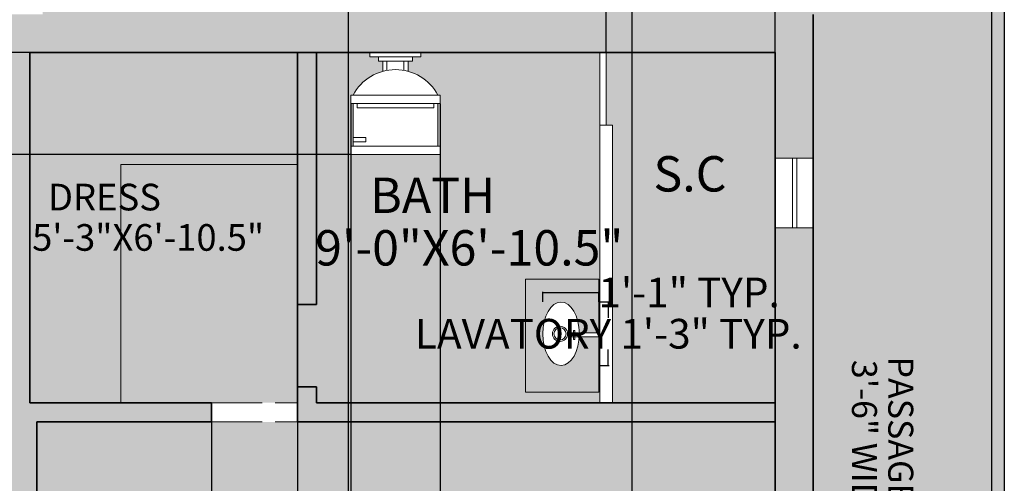
# Model space of a CAD drawing. Units: inches. Extents: x 1884 to 2398, y 474 to 1488.
# Tile 38 of 39: x 2165 to 2397, y 1233 to 1343. Entities that reach past the tile are written whole.
import ezdxf

# ---------------------------------------------------------------- set-up
doc = ezdxf.new("R2010")
doc.units = ezdxf.units.IN
doc.header["$MEASUREMENT"] = 0
doc.linetypes.add('ACAD_ISO02W100', pattern=[15, 12, -3])
doc.layers.get('0').update_dxf_attribs({"color": 250})
for name, color, linetype, lineweight in [('A-ANNO-DIMS', 2, 'Continuous', 18), ('A-AREA-IDEN', 7, 'Continuous', 18), ('A-FLOR-CASE', 8, 'Continuous', 20), ('A-FLOR-FIXT', 8, 'Continuous', 18), ('A-FLOR-OVHD', 8, 'ACAD_ISO02W100', 18), ('A-FLOR-PATT', 254, 'Continuous', 13), ('A-WALL-PATT', 250, 'Continuous', 13), ('C-PROP', 7, 'Continuous', 30), ('walls', 7, 'Continuous', 35), ('windows', 4, 'Continuous', 18)]:
    doc.layers.add(name, color=color, linetype=linetype, lineweight=lineweight)
doc.layers.add('A-FLOR-CASE-PATT', color=251, linetype='Continuous', lineweight=13, true_color=0x636466)
doc.layers.add('L-PVMT-PATT', color=9, linetype='Continuous', lineweight=13, true_color=0xc7c8ca)
doc.styles.get("Standard").update_dxf_attribs({"font": 'arial.ttf'})
doc.dimstyles.get("Standard").update_dxf_attribs({"dimtxt": 7, "dimasz": 0.18, "dimexe": 0.18, "dimexo": 0.0625, "dimgap": 0.09, "dimtad": 0, "dimtih": 1, "dimtoh": 1, "dimzin": 0, "dimdsep": 46, "dimlunit": 3, "dimtxsty": 'Standard', "dimcen": 0.09, "dimadec": 0, "dimazin": 0, "dimtfac": 1, "dimtofl": 0, "dimtmove": 0, "dimatfit": 3, "dimfxl": 1, "dimtolj": 1, "dimtzin": 0, "dimarcsym": 0})

# ---------------------------------------------------------------- blocks, each defined once
blk = doc.blocks.new('*U9')
for p, q in [((-10, 22), (-10, 12)), ((-10, 21), (-7, 21)), ((-7, 21), (-7, 20)), ((10, 12), (10, 22)), ((-7, 20), (-10, 20)), ((10.5, 12), (-10.5, 12)), ((-10.5, 10), (-10.5, 12)), ((9, 13), (-9, 13)), ((-9, 13), (-9, 12)), ((9, 12), (9, 13)), ((10.5, 12), (10.5, 10)), ((10.5, 10), (-10.5, 10)), ((-3, 4.406499999999937), (-3, 2)), ((-2, 2), (-2, 4.16579999999999)), ((2, 4.16579999999999), (2, 2)), ((3, 2), (3, 4.406499999999937)), ((4, 2), (-4, 2)), ((-4, 2), (-4, 1)), ((4, 1), (4, 2))]:
    blk.add_line(p, q)
for points in [[(10.5, 22), (10.5, 24), (-10.5, 24), (-10.5, 22)], [(6, 0), (6, 1), (-6, 1), (-6, 0)]]:
    blk.add_lwpolyline(points, close=True)
blk.add_arc((0, 15.33330000000001), 11.33333, 208.0725, 331.9275)
blk = doc.blocks.new('LAV-OVAL-WITH-TAP')
for p, q in [((7.274409562516666, 6.788668499560117), (7.274409562516666, 13.20873658643177)), ((8.219307397775992, 6.788668499560117), (8.219307397775992, 13.20873658643177)), ((6.697205447740998, 7.581094872117319), (8.82130564205363, 7.581094872117319)), ((6.69720544774077, 7.285663748863044), (6.697205447740998, 7.581094872117319)), ((8.82130564205363, 7.285663748863044), (6.69720544774077, 7.285663748863044)), ((8.82130564205363, 7.581094872117319), (8.82130564205363, 7.285663748863044)), ((7.274409562516666, 6.788668499560117), (8.219307397775992, 6.788668499560117))]:
    blk.add_line(p, q)
for radius in [1.786721855987963, 1.786721855987973, 1.426627914243592, 1.426627914243628, 1.42662769250472, 1.426627377330596]:
    blk.add_circle((7.497021151795252, 4.073758747890906), radius)
blk.add_ellipse((7.480663978300754, 4.312467997805015), major_axis=(-7.480193534640648, -0.0164125256646912), ratio=0.5765346257282574)
blk = doc.blocks.new('*D37')
at = {"layer": 'A-ANNO-DIMS', "color": 0, "lineweight": -2, "transparency": 16777216}
for p, q in [((2301.072042581748, 1276.125547417238), (2303.435168422141, 1276.125547417238)), ((2303.255168422141, 1275.945547417238), (2303.255168422141, 1272.354275288967)), ((2303.255168422141, 1261.334708481297), (2303.255168422141, 1264.925980609567)), ((2301.07204258175, 1261.154708481297), (2303.435168422141, 1261.154708481297))]:
    blk.add_line(p, q, dxfattribs=at)
at = {"layer": 'A-ANNO-DIMS', "color": 0, "lineweight": 100, "transparency": 16777216}
for points in [[(2303.225168422141, 1275.945547417238), (2303.285168422141, 1275.945547417238), (2303.255168422141, 1276.125547417238)], [(2303.225168422141, 1261.334708481297), (2303.285168422141, 1261.334708481297), (2303.255168422141, 1261.154708481297)]]:
    blk.add_solid(points, dxfattribs=at)
at = {"layer": 'Defpoints', "color": 0, "lineweight": 100, "transparency": 16777216}
for p in [(2301.009542581748, 1276.125547417238), (2301.009542581749, 1261.154708481297), (2303.255168422141, 1261.154708481297)]:
    blk.add_point(p, dxfattribs=at)
at = {"layer": 'A-ANNO-DIMS', "color": 0, "transparency": 16777216, "insert": (2303.255168422141, 1268.640127949266), "char_height": 7, "attachment_point": 5}
blk.add_mtext('\\A1;LAVATORY 1\'-3" TYP.', dxfattribs=at)
blk = doc.blocks.new('*D38')
at = {"layer": 'A-ANNO-DIMS', "color": 0, "lineweight": -2, "transparency": 16777216}
for p, q in [((2287.79161902562, 1276.188047417236), (2287.79161902562, 1278.551173257628)), ((2287.97161902562, 1278.371173257628), (2300.829542581747, 1278.371173257628)), ((2301.009542581747, 1276.188047417238), (2301.009542581747, 1278.551173257628)), ((2301.009542581747, 1278.371173257628), (2301.189542581747, 1278.371173257628))]:
    blk.add_line(p, q, dxfattribs=at)
at = {"layer": 'A-ANNO-DIMS', "color": 0, "lineweight": 100, "transparency": 16777216}
for points in [[(2287.97161902562, 1278.401173257628), (2287.97161902562, 1278.341173257628), (2287.79161902562, 1278.371173257628)], [(2300.829542581747, 1278.401173257628), (2300.829542581747, 1278.341173257628), (2301.009542581747, 1278.371173257628)]]:
    blk.add_solid(points, dxfattribs=at)
at = {"layer": 'Defpoints', "color": 0, "lineweight": 100, "transparency": 16777216}
for p in [(2301.009542581747, 1278.371173257628), (2287.79161902562, 1276.125547417236), (2301.009542581747, 1276.125547417238)]:
    blk.add_point(p, dxfattribs=at)
at = {"layer": 'A-ANNO-DIMS', "color": 0, "transparency": 16777216, "insert": (2322.284317479427, 1278.371173257628), "char_height": 7, "attachment_point": 5}
blk.add_mtext('\\A1;1\'-1" TYP.', dxfattribs=at)
blk = doc.blocks.new('*D43')
at = {"layer": 'A-ANNO-DIMS', "color": 0, "lineweight": -2, "transparency": 16777216}
for p, q in [((2302.732834, 1334.947237), (2302.732834, 1477.764705)), ((2302.912834, 1477.584705), (2313.239446317872, 1477.584705)), ((2342.34906, 1477.584705), (2332.022447682128, 1477.584705)), ((2342.52906, 1334.947237), (2342.52906, 1477.764705))]:
    blk.add_line(p, q, dxfattribs=at)
at = {"layer": 'A-ANNO-DIMS', "color": 0, "lineweight": 100, "transparency": 16777216}
for points in [[(2302.912834, 1477.614705), (2302.912834, 1477.554705), (2302.732834, 1477.584705)], [(2342.34906, 1477.614705), (2342.34906, 1477.554705), (2342.52906, 1477.584705)]]:
    blk.add_solid(points, dxfattribs=at)
at = {"layer": 'Defpoints', "color": 0, "lineweight": 100, "transparency": 16777216}
for p in [(2342.52906, 1477.584705), (2302.732834, 1334.884737), (2342.52906, 1334.884737)]:
    blk.add_point(p, dxfattribs=at)
at = {"layer": 'A-ANNO-DIMS', "color": 0, "transparency": 16777216, "insert": (2322.630947, 1477.584705), "char_height": 7, "attachment_point": 5}
blk.add_mtext('\\A1;3\'-4"', dxfattribs=at)
blk = doc.blocks.new('*D44')
at = {"layer": 'A-ANNO-DIMS', "color": 0, "lineweight": -2, "transparency": 16777216}
for p, q in [((2209.755415, 1247.822237), (2209.755415, 484.004737)), ((2230.02906, 1247.822237), (2230.02906, 484.004737)), ((2209.935415, 484.1847369999999), (2229.84906, 484.1847369999999)), ((2230.02906, 484.1847369999999), (2230.20906, 484.1847369999999))]:
    blk.add_line(p, q, dxfattribs=at)
at = {"layer": 'A-ANNO-DIMS', "color": 0, "lineweight": 100, "transparency": 16777216}
for points in [[(2209.935415, 484.2147369999999), (2209.935415, 484.1547369999999), (2209.755415, 484.1847369999999)], [(2229.84906, 484.2147369999999), (2229.84906, 484.1547369999999), (2230.02906, 484.1847369999999)]]:
    blk.add_solid(points, dxfattribs=at)
at = {"layer": 'Defpoints', "color": 0, "lineweight": 100, "transparency": 16777216}
for p in [(2209.755415, 1247.884737), (2230.02906, 1247.884737), (2230.02906, 484.1847369999999)]:
    blk.add_point(p, dxfattribs=at)
at = {"layer": 'A-ANNO-DIMS', "color": 0, "transparency": 16777216, "insert": (2247.429005429741, 484.1847369999999), "char_height": 7, "attachment_point": 5}
blk.add_mtext('\\A1;1\'-8 1/2"', dxfattribs=at)
blk = doc.blocks.new('*D45')
at = {"layer": 'A-ANNO-DIMS', "color": 0, "lineweight": -2, "transparency": 16777216}
for p, q in [((2242.616569, 1322.822237), (2242.616569, 484.004737)), ((2263.616569, 1322.822237), (2263.616569, 484.004737)), ((2242.796569, 484.1847369999999), (2244.052148809004, 484.1847369999999)), ((2263.436569, 484.1847369999999), (2262.180989190996, 484.1847369999999))]:
    blk.add_line(p, q, dxfattribs=at)
at = {"layer": 'A-ANNO-DIMS', "color": 0, "lineweight": 100, "transparency": 16777216}
for points in [[(2242.796569, 484.2147369999999), (2242.796569, 484.1547369999999), (2242.616569, 484.1847369999999)], [(2263.436569, 484.2147369999999), (2263.436569, 484.1547369999999), (2263.616569, 484.1847369999999)]]:
    blk.add_solid(points, dxfattribs=at)
at = {"layer": 'Defpoints', "color": 0, "lineweight": 100, "transparency": 16777216}
for p in [(2242.616569, 1322.884737), (2263.616569, 1322.884737), (2263.616569, 484.1847369999999)]:
    blk.add_point(p, dxfattribs=at)
at = {"layer": 'A-ANNO-DIMS', "color": 0, "transparency": 16777216, "insert": (2253.116569, 484.1847369999999), "char_height": 7, "attachment_point": 5}
blk.add_mtext('\\A1;1\'-9"', dxfattribs=at)
blk = doc.blocks.new('*D46')
at = {"layer": 'A-ANNO-DIMS', "color": 0, "lineweight": -2, "transparency": 16777216}
for p, q in [((2247.054069000001, 1334.884737), (1902.431692000002, 1334.884737)), ((1902.611692000002, 1334.704737), (1902.611692000002, 1326.548747914052)), ((1902.611692000002, 1311.064737), (1902.611692000002, 1319.220726085948)), ((2242.554069000001, 1310.884737), (1902.431692000002, 1310.884737))]:
    blk.add_line(p, q, dxfattribs=at)
at = {"layer": 'A-ANNO-DIMS', "color": 0, "lineweight": 100, "transparency": 16777216}
for points in [[(1902.581692000002, 1334.704737), (1902.641692000002, 1334.704737), (1902.611692000002, 1334.884737)], [(1902.581692000002, 1311.064737), (1902.641692000002, 1311.064737), (1902.611692000002, 1310.884737)]]:
    blk.add_solid(points, dxfattribs=at)
at = {"layer": 'Defpoints', "color": 0, "lineweight": 100, "transparency": 16777216}
for p in [(2247.116569000001, 1334.884737), (1902.611692000002, 1310.884737), (2242.616569000001, 1310.884737)]:
    blk.add_point(p, dxfattribs=at)
at = {"layer": 'A-ANNO-DIMS', "color": 0, "transparency": 16777216, "insert": (1902.611692000002, 1322.884737), "char_height": 7, "attachment_point": 5}
blk.add_mtext('\\A1;2\'-0"', dxfattribs=at)
blk = doc.blocks.new('*D52')
at = {"layer": 'A-ANNO-DIMS', "color": 0, "lineweight": -2, "transparency": 16777216}
for p, q in [((2308.845502, 820.8887220000001), (2308.845502, 1477.764705)), ((2309.025502, 1477.584705), (2342.34906, 1477.584705)), ((2342.52906, 820.8887220000001), (2342.52906, 1477.764705)), ((2342.52906, 1477.584705), (2342.70906, 1477.584705))]:
    blk.add_line(p, q, dxfattribs=at)
at = {"layer": 'A-ANNO-DIMS', "color": 0, "lineweight": 100, "transparency": 16777216}
for points in [[(2309.025502, 1477.614705), (2309.025502, 1477.554705), (2308.845502, 1477.584705)], [(2342.34906, 1477.614705), (2342.34906, 1477.554705), (2342.52906, 1477.584705)]]:
    blk.add_solid(points, dxfattribs=at)
at = {"layer": 'Defpoints', "color": 0, "lineweight": 100, "transparency": 16777216}
for p in [(2342.52906, 1477.584705), (2308.845502, 820.8262219999999), (2342.52906, 820.8262219999999)]:
    blk.add_point(p, dxfattribs=at)
at = {"layer": 'A-ANNO-DIMS', "color": 0, "transparency": 16777216, "insert": (2360.318159590723, 1477.584705), "char_height": 7, "attachment_point": 5}
blk.add_mtext('\\A1;2\'-9 1/2"', dxfattribs=at)
blk = doc.blocks.new('*D54')
at = {"layer": 'A-ANNO-DIMS', "color": 0, "lineweight": -2, "transparency": 16777216}
for p, q in [((2242.059232, 893.028555), (2242.059232, 1477.764705)), ((2242.239232, 1477.584705), (2266.058478869031, 1477.584705)), ((2308.665502, 1477.584705), (2284.846255130969, 1477.584705)), ((2308.845502, 893.028555), (2308.845502, 1477.764705))]:
    blk.add_line(p, q, dxfattribs=at)
at = {"layer": 'A-ANNO-DIMS', "color": 0, "lineweight": 100, "transparency": 16777216}
for points in [[(2242.239232, 1477.614705), (2242.239232, 1477.554705), (2242.059232, 1477.584705)], [(2308.665502, 1477.614705), (2308.665502, 1477.554705), (2308.845502, 1477.584705)]]:
    blk.add_solid(points, dxfattribs=at)
at = {"layer": 'Defpoints', "color": 0, "lineweight": 100, "transparency": 16777216}
for p in [(2308.845502, 1477.584705), (2242.059232, 892.9660549999999), (2308.845502, 892.9660549999999)]:
    blk.add_point(p, dxfattribs=at)
at = {"layer": 'A-ANNO-DIMS', "color": 0, "transparency": 16777216, "insert": (2275.452367, 1477.584705), "char_height": 7, "attachment_point": 5}
blk.add_mtext('\\A1;5\'-7"', dxfattribs=at)

msp = doc.modelspace()

# ---------------------------------------------------------------- hatches: boundary and pattern name
at = {"layer": 'A-FLOR-CASE-PATT'}
h = msp.add_hatch(color=256, dxfattribs=at)
h.dxf.hatch_style = 1
h.paths.add_polyline_path([(2230.029060307534, 1334.884736586432), (2167.029060307534, 1334.884736586432), (2167.029060307533, 1252.384736586432), (2188.39223788629, 1252.384736586432), (2188.39223788629, 1308.548092360888), (2230.029060307534, 1308.548092360888)])
h.paths.add_polyline_path([(2087.529060307534, 1341.419208402589), (2019.112052587603, 1341.419208402589), (2019.112052587603, 1327.384736586431), (2019.112052587603, 1322.884736586432), (2087.529060307534, 1322.884736586431)])
h = msp.add_hatch(color=256, dxfattribs=at)
h.dxf.hatch_style = 1
edge = h.paths.add_edge_path()
edge.add_line((2301.009542581749, 1268.846382365051), (2301.009542581749, 1281.541714860787))
edge.add_line((2301.009542581749, 1281.541714860787), (2283.754419727821, 1281.541714860787))
edge.add_line((2283.754419727821, 1281.541714860787), (2283.754419727821, 1254.895307848658))
edge.add_line((2283.754419727821, 1254.895307848658), (2301.009542581749, 1254.895307848658))
edge.add_line((2301.009542581749, 1254.895307848658), (2301.009542581749, 1267.901484529792))
edge.add_line((2301.009542581749, 1267.901484529792), (2296.405886518651, 1267.901484529792))
edge.add_ellipse((2292.113273993122, 1268.640127949267), major_axis=(-0.0164125256646898, 7.480193534640648), ratio=0.5765346257282575, start_angle=272.6136539907866, end_angle=620.1108329880406, ccw=False)
edge.add_line((2296.423940027922, 1268.846382365051), (2301.009542581749, 1268.846382365051))
at = {"layer": 'A-FLOR-PATT'}
h = msp.add_hatch(color=256, dxfattribs=at)
h.dxf.hatch_style = 1
h.paths.add_polyline_path([(2050.106778681225, 1363.349576779681), (2050.106778681225, 1397.884736586431), (2042.590228763987, 1397.884736586431), (2042.590228763987, 1396.884736586432), (2040.590228763988, 1396.884736586432), (2040.590228763988, 1395.884736586431), (2039.590228763987, 1395.884736586431), (2039.590228763987, 1393.480497336967, -0.2060810176159205), (2046.590242763922, 1387.884736586431), (2047.090228763988, 1387.884736586431), (2047.090228763988, 1385.884736586431), (2046.590228763987, 1385.884736586431), (2046.590228763987, 1375.884736586432), (2047.090228763988, 1375.884736586432), (2047.090228763988, 1373.884736586431), (2026.090228763988, 1373.884736586431), (2026.090228763988, 1375.884736586432), (2026.590228763987, 1375.884736586432), (2026.590228763987, 1385.884736586431), (2026.090228763988, 1385.884736586431), (2026.090228763988, 1387.884736586431), (2026.590214764052, 1387.884736586431, -0.2060810176159205), (2033.590228763987, 1393.480497336967), (2033.590228763987, 1395.884736586431), (2032.590228763988, 1395.884736586431), (2032.590228763988, 1396.884736586432), (2030.590228763987, 1396.884736586432), (2030.590228763987, 1397.884736586431), (1990.41848407891, 1397.884736586431), (1990.418484078909, 1380.629613732504), (1963.77207706678, 1380.629613732504), (1963.77207706678, 1397.884736586431), (1961.529060307533, 1397.884736586431), (1961.529060307533, 1327.560779427295), (1965.065804798096, 1327.560779427295), (1965.065804798096, 1322.884736586432), (2007.131770728449, 1322.884736586432), (2007.131770728449, 1327.384736586431), (2014.612052587603, 1327.384736586431), (2014.612052587603, 1345.919208402589), (2050.106778681225, 1345.919208402589)])
h.paths.add_polyline_path([(2087.529060307534, 1397.884736586431), (2053.062200912405, 1397.884736586431), (2053.062200912405, 1363.349576779681), (2051.584489796816, 1363.349576779681), (2051.584489796816, 1345.919208402589), (2087.529060307534, 1345.919208402589)])
h.paths.add_polyline_path([(2301.255122477188, 1334.884736586432), (2265.892029109202, 1334.884736586432), (2259.116568963785, 1334.884736586432), (2259.116568963785, 1333.884736586432), (2257.116568963786, 1333.884736586432), (2257.116568963786, 1332.884736586432), (2256.116568963786, 1332.884736586432), (2256.116568963786, 1330.480497336967, -0.2060810176159197), (2263.116582963721, 1324.884736586432), (2263.616568963786, 1324.884736586432), (2263.616568963786, 1322.884736586432), (2263.116568963786, 1322.884736586432), (2263.116568963786, 1312.884736586432), (2263.616568963786, 1312.884736586432), (2263.616568963786, 1310.884736586432), (2242.616568963786, 1310.884736586432), (2242.616568963786, 1312.884736586432), (2243.116568963785, 1312.884736586432), (2243.116568963785, 1322.884736586432), (2242.616568963786, 1322.884736586432), (2242.616568963786, 1324.884736586432), (2243.11655496385, 1324.884736586432, -0.2060810176159197), (2250.116568963786, 1330.480497336967), (2250.116568963786, 1332.884736586432), (2249.116568963786, 1332.884736586432), (2249.116568963786, 1333.884736586432), (2247.116568963786, 1333.884736586432), (2247.116568963786, 1334.884736586432), (2234.529060307534, 1334.884736586432), (2234.529060307533, 1275.553826810391), (2230.029060307533, 1275.553826810391), (2230.029060307533, 1256.117249027531), (2234.529060307533, 1256.117249027531), (2234.529060307533, 1252.384736586432), (2265.892029109202, 1252.384736586432), (2301.255122477188, 1252.384736586432)])
h.paths.add_polyline_path([(2283.754419727821, 1281.541714860787), (2301.009542581749, 1281.541714860787), (2301.009542581749, 1254.895307848658), (2283.754419727821, 1254.895307848658)], flags=16)
edge = h.paths.add_edge_path(flags=0)
edge.add_ellipse((2292.113273993122, 1268.640127949267), major_axis=(-0.0164125256646898, 7.480193534640649), ratio=0.5765346257282574, start_angle=272.6136539907895, end_angle=620.1108329880437, ccw=False)
edge.add_ellipse((2292.113273993122, 1268.640127949267), major_axis=(-0.0164125256646898, 7.480193534640649), ratio=0.5765346257282574, start_angle=260.1108329880437, end_angle=272.6136539907895, ccw=False)
h.paths.add_polyline_path([(2293.661286599196, 1268.623770775773, -1), (2290.08784288722, 1268.623770775773, -1)], flags=0)
h.paths.add_polyline_path([(2290.447937365877, 1268.623770775773, -1), (2293.301192120539, 1268.623770775773, -1)], flags=0)
h.paths.add_polyline_path([(2295.08646974418, 1269.423586479827), (2295.381900867434, 1269.423586479827), (2295.381900867434, 1267.299486285514), (2295.08646974418, 1267.299486285514), (2295.08646974418, 1267.901484529792), (2294.589474494877, 1267.901484529792), (2294.589474494877, 1268.846382365051), (2295.08646974418, 1268.846382365051)], flags=0)
h.paths.add_polyline_path([(2342.529060307533, 1334.884736586432), (2302.732833592778, 1334.884736586432), (2302.732833592777, 1317.822173990474), (2304.210544708368, 1317.822173990474), (2304.210544708368, 1252.384736586432), (2342.529060307533, 1252.384736586432), (2342.529060307533, 1276.19700522134)])
h = msp.add_hatch(color=256, dxfattribs=at)
h.dxf.hatch_style = 1
h.paths.add_polyline_path([(2117.529060307534, 815.8008601642414), (2126.529060307533, 815.8008601642414), (2126.529060307534, 880.3823245284138), (2117.529060307534, 880.3823245284138), (2117.529060307534, 892.3847365864315), (1961.529060307533, 892.3847365864318), (1961.529060307533, 756.9152132436575), (1964.529060307533, 756.9152132436575), (1964.529060307533, 759.9152132436574), (1995.529060307533, 759.9152132436574), (1995.529060307533, 753.9152132436575), (1972.862393640866, 753.9152132436575), (1967.529060307533, 756.9152132436575), (1967.529060307533, 654.9152132436574), (1972.862393640866, 657.9152132436575), (1995.529060307533, 657.9152132436575), (1995.529060307533, 651.9152132436574), (1964.529060307533, 651.9152132436574), (1964.529060307533, 654.9152132436574), (1961.529060307533, 654.9152132436574), (1961.529060307533, 640.3847365864318), (2117.529060307534, 640.3847365864314), (2117.529060307534, 646.5776756488413), (2126.529060307534, 646.5776756488413), (2126.529060307533, 676.1826019380942), (2117.529060307534, 676.1826019380942)])
h.paths.add_polyline_path([(2012.245892997025, 808.9291988189563), (2012.049579081969, 810.1854570579605), (2032.542313208683, 810.1854570579605), (2032.346024821094, 808.9291988189563)], flags=16)
h.paths.add_polyline_path([(2010.38119353609, 820.8636520894975), (1994.658277650963, 820.8636520894975), (1994.658277650963, 831.5614635913172), (1984.608211738929, 833.1317793251212), (1984.608211738929, 853.8208002572304), (1994.658277650963, 855.3911120678468), (1994.658277650963, 866.0889486936543), (2010.381193536673, 866.0889486936543), (2011.951435886253, 876.1390146056889), (2032.640472118199, 876.1390146056889), (2034.210849866988, 866.0889486936543), (2045.556424228796, 866.0889486936543), (2047.126666578375, 876.1390146056889), (2067.815702810321, 876.1390146056889), (2069.386080559109, 866.0889486936543), (2085.108870859277, 866.0889486936543), (2085.108870859277, 855.3911120678468), (2095.158936771312, 853.8208002572304), (2095.158936771312, 833.1317793251212), (2085.108870859277, 831.5614635913172), (2085.108870859277, 820.8636520894975), (2069.386080560277, 820.8636520894975), (2067.815706736618, 810.8135861774629), (2047.126664615719, 810.8135861774629), (2045.556424228212, 820.8636520894975), (2034.210849868156, 820.8636520894975), (2032.640476044496, 810.8135861774629), (2011.951433923597, 810.8135861774629)], flags=16)
h.paths.add_polyline_path([(1982.723824380422, 833.426234479541), (1982.723824380422, 853.5263663036108), (1983.980082619426, 853.7226346601389), (1983.980082619426, 833.2299276462522)], flags=16)
h.paths.add_polyline_path([(1994.529060307533, 753.5402132436574), (1994.529060307533, 658.2902132436575), (1973.529060307533, 658.2902132436575), (1973.529060307533, 753.5402132436574)], flags=16)
h.paths.add_polyline_path([(2084.48576677273, 843.5274175393209), (2084.59204621975, 843.5024682506945), (2084.680989303072, 843.4873429014967), (2084.812983397052, 843.4769081193547), (2084.91314582564, 843.4767023942125), (2084.66880953484, 843.4819332556493), (2084.336020790642, 843.5646279083602), (2084.11630122464, 843.6165616239609), (2083.80035227753, 843.6856683896884), (2083.105016757222, 843.8265189249884), (2082.836048453269, 843.873780498397), (2083.603851506107, 843.7286485385392), (2084.20582336258, 843.5969806585211)], flags=0)
h.paths.add_polyline_path([(2047.421123689146, 808.9291988189563), (2047.224809774091, 810.1854570579605), (2067.717543900804, 810.1854570579605), (2067.521255513216, 808.9291988189563)], flags=16)
h.paths.add_polyline_path([(2066.009851225869, 849.5050711179754), (2066.42856209693, 849.6872536877958), (2066.798278896669, 849.8816973380289), (2067.128674813528, 850.0847337946167), (2067.429674287593, 850.2926822209193), (2067.71107613313, 850.501861780296), (2068.176225202245, 850.8560509488422), (2068.688503010997, 851.2051162670248), (2069.305475594623, 851.5305287965867), (2070.015309134756, 851.783837036287), (2070.843781436505, 851.9440833228273), (2071.080737607611, 851.9560435048553), (2070.628610267393, 851.9024640909616), (2070.212160661163, 851.8219128126768), (2069.82749438838, 851.7168142484016), (2069.471093925975, 851.5896306642849), (2069.13919049923, 851.4428243264747), (2068.828266585076, 851.2788323759551), (2068.534427782973, 851.1001296414569), (2068.254156569851, 850.9091532639633), (2067.982553538579, 850.708579073524), (2067.501844470646, 850.3425416967154), (2066.951193479014, 849.9621190813364), (2066.223646961128, 849.579483505263)], flags=0)
h.paths.add_polyline_path([(2059.423038027123, 853.2214975541691), (2059.826673799315, 853.277727672947), (2060.171391060097, 853.3584925151328), (2060.464601733081, 853.462573510234), (2060.713717741875, 853.5887269625948), (2060.925899758443, 853.7357343017233), (2061.107303448155, 853.9021759558088), (2061.257928811012, 854.0857906600216), (2061.376770840422, 854.2841287107957), (2061.462447652322, 854.4947278419824), (2061.513828614297, 854.7151509125981), (2061.529531842285, 854.9429230939121), (2061.508426703869, 855.1756072449404), (2061.449382566637, 855.4107536621171), (2061.352399430585, 855.6463020819306), (2061.223632961088, 855.8818505017439), (2061.070243830105, 856.1173989215573), (2060.899769587072, 856.3529473413709), (2060.719370903951, 856.588495761183), (2060.405833605864, 856.9925386710904), (2060.102852609014, 857.4235624716171), (2059.858108421559, 857.8880530440814), (2059.691164532255, 858.4673451479222), (2059.835525259983, 859.0912752050886), (2060.304837982534, 859.5324417717479), (2060.843952795028, 859.7984964546366), (2061.512696715463, 859.9353091544514), (2062.253367096678, 859.9051905068), (2062.482906219865, 859.8492647715083), (2062.077511686138, 859.9123414976887), (2061.695357929833, 859.9278814121051), (2061.33644495095, 859.8992512868383), (2061.004667150029, 859.8313756541849), (2060.703416424316, 859.7291413586948), (2060.436587174351, 859.5974603700822), (2060.207822549028, 859.4412446580619), (2060.020765697241, 859.2654061923486), (2059.879059767881, 859.0748318174917), (2059.785217277427, 858.8738430618334), (2059.736725709402, 858.6642614998202), (2059.729941914911, 858.4473182645266), (2059.761222745062, 858.2242444890267), (2059.826925050962, 857.9962587438123), (2059.92315443207, 857.7646047245396), (2060.04651899114, 857.5304758765365), (2060.193124327632, 857.2951410206236), (2060.358699163532, 857.0595926008104), (2060.536585330176, 856.8240441809971), (2060.866718458323, 856.3986148921463), (2061.170885250692, 855.9783402158826), (2061.422381845951, 855.5182854684566), (2061.56688892396, 854.942778343735), (2061.410468633091, 854.271739120365), (2060.947138393936, 853.7069322166539), (2060.334567557683, 853.3967236267573), (2059.649288497294, 853.2361675378636)], flags=0)
h.paths.add_polyline_path([(2050.777720077942, 859.7454978409666), (2051.07042824763, 859.870219158935), (2051.294544717468, 860.017025496745), (2051.46690334786, 860.1832661495123), (2051.593911055823, 860.3654487193328), (2051.679210990252, 860.5598923695659), (2051.726446300039, 860.7629288261536), (2051.739260134076, 860.9708772524561), (2051.721546892906, 861.1800568118329), (2051.676698473774, 861.386774105061), (2051.60860927722, 861.5873482955004), (2051.521299329609, 861.7789402395308), (2051.420547418841, 861.9619393772065), (2051.312383584462, 862.1375768416017), (2051.202963491846, 862.3070837657913), (2050.966442536983, 862.6795474136981), (2050.793480878491, 863.1925713661464), (2051.021372914674, 863.6992722615545), (2051.482558609153, 864.0178750295152), (2052.090482216228, 864.1376203451599), (2052.773111098533, 864.157049396074), (2053.006824697232, 864.1424016774818), (2052.60318892504, 864.1522130543284), (2052.258471664257, 864.1424016774818), (2051.965260991273, 864.1129549843595), (2051.716144982478, 864.063885537544), (2051.50396296591, 863.9951807744528), (2051.322433650375, 863.907255260305), (2051.170300777631, 863.8021566960299), (2051.04756434768, 863.6823473477759), (2050.954349986346, 863.5502517939447), (2050.890532067805, 863.4083574258491), (2050.85623621788, 863.2590888218906), (2050.851336810748, 863.1049208108001), (2050.875833846408, 862.9483030961434), (2050.928847944094, 862.7910572523672), (2051.005102819202, 862.6326054006817), (2051.09844280636, 862.4716787202652), (2051.202963491844, 862.3070837657904), (2051.312383584462, 862.1375768416013), (2051.556251316974, 861.7415820950013), (2051.751339156135, 861.1669008329959), (2051.712429226858, 860.5354537160036), (2051.398466566313, 860.0850989679107), (2050.948595340801, 859.7904131416026)], flags=0)
h.paths.add_polyline_path([(2022.768265091874, 719.2635269564156), (2050.460701888225, 719.2635269564156), (2050.460701888225, 717.2264308545614), (2052.426027545829, 717.2264308545614), (2052.426027545829, 715.0328555474166), (2050.460701888225, 715.0328555474166), (2050.460701888225, 703.7384712949378), (2022.768265091874, 703.7384712949378)], flags=16)
h.paths.add_polyline_path([(2012.245892997025, 878.0234019641955), (2032.346024821094, 878.0234019641955), (2032.542311246466, 876.7671437251912), (2012.049583009897, 876.7671437251912)], flags=16)
h.paths.add_polyline_path([(2035.324314229629, 713.1026297220419), (2035.342323734454, 713.2939269647811), (2035.191594480285, 713.2022463391573)], flags=0)
h.paths.add_polyline_path([(2036.483793368253, 711.6303552235653), (2036.583057308503, 711.849035191806), (2036.389574164252, 711.8976249102717)], flags=0)
h.paths.add_polyline_path([(2036.073963013272, 712.7444251806157), (2035.992966259493, 712.4813789411762), (2035.723718538195, 712.5164991793641), (2035.794480886751, 712.7255350820222)], flags=0)
h.paths.add_polyline_path([(2035.845889740907, 710.9094011156075), (2035.752657170415, 710.9579395480923), (2035.701796841489, 710.8802910191051)], flags=0)
h.paths.add_polyline_path([(2037.817833105062, 712.0186444527698), (2037.94771907015, 712.060054181353), (2037.986590761345, 712.1613470938162), (2037.815493232997, 712.0195830652098)], flags=0)
h.paths.add_polyline_path([(2038.451438253888, 709.5174527548473), (2038.46381259532, 709.4275335183239), (2038.585708407037, 709.4415430414689)], flags=0)
h.paths.add_polyline_path([(2037.805223875722, 709.8056815263456), (2037.818420097464, 709.807253189157), (2037.804492020793, 709.8227772356641)], flags=0)
h.paths.add_polyline_path([(2036.699670737428, 711.2453724121245), (2036.698482732612, 711.2358968812113), (2036.813156202547, 711.2113760065187)], flags=0)
h.paths.add_polyline_path([(2035.92842163957, 708.8974795736603), (2035.668252200497, 708.8712447892582), (2035.705968573039, 708.6672524113528)], flags=0)
h.paths.add_polyline_path([(2036.4135388155, 710.9761633445361), (2035.932343572741, 709.8585852823189), (2036.792006299979, 710.4843975690396), (2036.499859551577, 710.934168748562)], flags=0)
h.paths.add_polyline_path([(2038.297960372458, 712.1148420018311), (2038.498945749665, 712.0579037604177), (2038.612442111864, 712.268650843707), (2038.390256576993, 712.3323300722286)], flags=0)
h.paths.add_polyline_path([(2047.421123689146, 878.0234019641955), (2067.521255513216, 878.0234019641955), (2067.717541938588, 876.7671437251912), (2047.224813702019, 876.7671437251912)], flags=16)
h.paths.add_polyline_path([(2049.647427742059, 705.0928292249858, -1), (2048.84548899896, 705.0928292249858, -1)], flags=0)
h.paths.add_polyline_path([(2095.787065890814, 853.7226542967927), (2097.043324129819, 853.5263663036108), (2097.043324129819, 833.426234479541), (2095.787065890814, 833.2299276462522)], flags=16)
h.paths.add_polyline_path([(2110.738728909887, 745.3388006828269), (2111.750023094465, 745.3388006828269, -0.0640418572917222), (2113.266964371214, 742.919542441155), (2113.266964371214, 732.1919762839284), (2113.525533380085, 732.1919762839282, -0.4142135623731062), (2114.278258555744, 731.4392511082686), (2114.278258555744, 716.7639945070974, -0.4142135623730951), (2113.525533380085, 716.0112693314378), (2113.266964371214, 716.0112693314377), (2113.266964371214, 705.2837031743313, -0.0640418572952104), (2111.750023094367, 702.8644449325391), (2110.738728909887, 702.8644449325391), (2110.738728909887, 716.0112693314377), (2109.468865716485, 716.0112693314378, -0.4142135623730951), (2108.716140540826, 716.7639945070974), (2108.716140540826, 731.4392511082686, -0.4142135623730951), (2109.468865716485, 732.1919762839282), (2110.738728909887, 732.1919762839284)], flags=16)
h.paths.add_polyline_path([(1998.045441111793, 668.9094387650339), (2002.449119404415, 668.9094387650339), (2002.449119404415, 652.2733207706847), (2002.724349297704, 652.762618358754), (2002.724349297704, 668.1754923829302), (2019.972089277139, 668.1754923829302), (2019.972089277139, 652.762618358754), (2020.247319170428, 652.2733207706847), (2020.247319170428, 668.9094387650339), (2024.65099746305, 668.9094387650339), (2029.054675755671, 668.9094387650334), (2029.054675755671, 652.2733207706846), (2029.329905648959, 652.7626183587535), (2029.32990564896, 668.1754923829299), (2046.577645628395, 668.1754923829296), (2046.577645628395, 652.7626183587535), (2046.852875521684, 652.2733207706846), (2046.852875521684, 668.9094387650333), (2051.256553814306, 668.9094387650332), (2051.256553814305, 646.1571009198206), (2049.054714667995, 646.1571009198207), (2049.054714667995, 643.9552617735098), (2026.85283660936, 643.9552617735101), (2026.85283660936, 646.157100919821), (2024.650997463049, 646.157100919821), (2022.449158316739, 646.1571009198213), (2022.449158316739, 643.9552617735103), (2000.247280258104, 643.9552617735103), (2000.247280258104, 646.1571009198213), (1998.045441111793, 646.1571009198213)], flags=16)
h.paths.add_polyline_path([(2342.529060307532, 1247.884736586432), (2265.892029109202, 1247.884736586432), (2230.029060307533, 1247.884736586432), (2209.755415465046, 1247.884736586432), (2168.600168546053, 1247.884736586432), (2168.600168546053, 1104.929335189726), (2158.029060307534, 1104.929335189726), (2158.029060307534, 1079.411493140081), (2168.600168546053, 1079.411493140081), (2168.600168546053, 1062.466054843048), (2342.529060307534, 1062.466054843048), (2342.529060307535, 1093.80946809509)])
h.paths.add_polyline_path([(2215.029585767078, 1153.875922220359), (2215.029585767078, 1164.738901046202), (2187.558514037159, 1164.738901046202), (2187.441848177233, 1152.640560104242), (2173.567560328407, 1152.640560104242), (2173.684226188333, 1164.738901046178), (2173.684226188333, 1218.738896358896), (2173.80089204826, 1230.837237300835), (2187.675179897085, 1230.837237300835), (2187.558514037159, 1218.738896358897), (2215.029585767078, 1218.738896358897), (2215.029585767078, 1225.878851812398), (2245.053154048409, 1225.878851812398), (2245.053154048409, 1153.875922220359)], flags=16)
h.paths.add_polyline_path([(2192.146797479106, 1164.797089366358), (2184.963183514796, 1174.540018628516), (2184.914853464182, 1174.540018628516), (2176.755013122293, 1174.540018628516), (2176.755013122293, 1190.362773833876), (2184.914853464182, 1190.362773833876), (2184.914853464182, 1196.818536437712), (2176.755013122293, 1196.818536437712), (2176.755013122293, 1212.641291643072), (2184.914853464182, 1212.641291643072), (2184.914853464182, 1174.605567287827), (2184.963183514796, 1174.540018628516), (2192.146797479106, 1174.540018628516)], flags=0)
h.paths.add_polyline_path([(2184.970820652961, 1158.363900966234, -1), (2176.038587852678, 1158.363900966234, -1)], flags=0)
h.paths.add_polyline_path([(2335.555222872957, 1161.985357442079), (2335.555222872957, 1175.132181840978), (2334.285359679555, 1175.132181840978, -0.4142135623730951), (2333.532634503896, 1175.884907016637), (2333.532634503896, 1190.560163617809, -0.4142135623730951), (2334.285359679555, 1191.312888793468), (2335.555222872957, 1191.312888793468), (2335.555222872957, 1204.459713192367), (2336.566517057534, 1204.459713192367, -0.0640418572917234), (2338.083458334283, 1202.040454950695), (2338.083458334283, 1191.312888793468), (2338.342027343154, 1191.312888793468, -0.4142135623731616), (2339.094752518814, 1190.560163617809), (2339.094752518814, 1175.884907016637, -0.4142135623730951), (2338.342027343154, 1175.132181840978), (2338.083458334283, 1175.132181840978), (2338.083458334283, 1164.404615683871, -0.0640418572952083), (2336.566517057436, 1161.985357442079)], flags=16)
h.paths.add_polyline_path([(2176.155253712605, 1224.462237220889, -1), (2185.087486512887, 1224.462237220889, -1)], flags=0)
h.paths.add_polyline_path([(2158.029060307534, 1276.19700522134), (2158.029060307534, 1322.884736586431), (2148.233210584229, 1322.884736586431), (2092.029060307534, 1322.884736586431), (1961.529060307533, 1322.884736586432), (1961.529060307533, 1166.884736586432), (2116.004926061792, 1166.884736586431), (2116.004926061792, 1157.884736586431), (2152.637676873365, 1157.884736586431), (2152.637676873365, 1166.884736586431), (2158.029060307534, 1166.884736586431)])
h.paths.add_polyline_path([(2006.351794059088, 1204.245313711267), (2006.351794059088, 1215.108292537111), (1978.880722329168, 1215.108292537111), (1978.764056469242, 1203.00995159515), (1964.889768620417, 1203.00995159515), (1965.006434480343, 1215.108292537088), (1965.006434480343, 1269.108287849805), (1965.123100340269, 1281.206628791743), (1978.997388189094, 1281.206628791743), (1978.880722329168, 1269.108287849805), (2006.351794059088, 1269.108287849805), (2006.351794059088, 1276.248243303306), (2036.375362340419, 1276.248243303306), (2036.375362340419, 1204.245313711267)], flags=16)
h.paths.add_polyline_path([(1983.469005771116, 1215.166480857267), (1976.285391806805, 1224.909410119424), (1976.237061756191, 1224.909410119424), (1968.077221414302, 1224.909410119424), (1968.077221414302, 1240.732165324784), (1976.237061756191, 1240.732165324784), (1976.237061756191, 1247.18792792862), (1968.077221414302, 1247.18792792862), (1968.077221414302, 1263.01068313398), (1976.237061756191, 1263.01068313398), (1976.237061756191, 1224.974958778736), (1976.285391806805, 1224.909410119424), (1983.469005771116, 1224.909410119424)], flags=0)
h.paths.add_polyline_path([(1976.293028944971, 1208.733292457142, -1), (1967.360796144688, 1208.733292457142, -1)], flags=0)
h.paths.add_polyline_path([(1967.477462004614, 1274.831628711797, -1), (1976.409694804897, 1274.831628711797, -1)], flags=0)
h.paths.add_polyline_path([(2152.586710801799, 1223.485042164994), (2152.586710801799, 1236.631866563892), (2151.316847608397, 1236.631866563892, -0.4142135623730951), (2150.564122432737, 1237.384591739552), (2150.564122432737, 1252.059848340723, -0.4142135623730951), (2151.316847608397, 1252.812573516383), (2152.586710801799, 1252.812573516383), (2152.586710801799, 1265.959397915281), (2153.598004986376, 1265.959397915281, -0.0640418572917215), (2155.114946263125, 1263.54013967361), (2155.114946263125, 1252.812573516383), (2155.373515271996, 1252.812573516383, -0.4142135623730288), (2156.126240447656, 1252.059848340723), (2156.126240447656, 1237.384591739552, -0.4142135623730951), (2155.373515271996, 1236.631866563892), (2155.114946263125, 1236.631866563892), (2155.114946263125, 1225.904300406786, -0.0640418572952094), (2153.598004986278, 1223.485042164994)], flags=16)
h.paths.add_polyline_path([(2250.676094667158, 1161.100728645635), (2322.077457416915, 1161.100728645635), (2322.077457416915, 1173.885720445675), (2250.676094667158, 1173.885720445675)], flags=24)
h.paths.add_polyline_path([(2255.610417877832, 1173.711980483038), (2320.135651303891, 1173.711980483038), (2320.135651303891, 1186.659131725134), (2255.610417877832, 1186.659131725134)], flags=24)
h.paths.add_polyline_path([(2053.687197260262, 1230.837005449875), (2125.088560010019, 1230.837005449875), (2125.088560010019, 1243.621997249915), (2053.687197260262, 1243.621997249915)], flags=24)
h.paths.add_polyline_path([(2058.621520470935, 1243.448257287277), (2123.146753896995, 1243.448257287277), (2123.146753896995, 1256.395408529374), (2058.621520470935, 1256.395408529374)], flags=24)
h = msp.add_hatch(color=256, dxfattribs=at)
h.dxf.hatch_style = 1
h.paths.add_polyline_path([(2230.029060307534, 1308.548092360888), (2188.39223788629, 1308.548092360888), (2188.39223788629, 1252.384736586432), (2209.755415465046, 1252.384736586432), (2230.029060307533, 1252.384736586432)])
h.paths.add_polyline_path([(2165.932414693997, 1286.482376901261), (2222.121748845521, 1286.482376901261), (2222.121748845521, 1296.107124106511), (2165.932414693997, 1296.107124106511)], flags=9)
h.paths.add_polyline_path([(2169.648123316137, 1295.977400715826), (2203.118428016548, 1295.977400715826), (2203.118428016548, 1305.717799089097), (2169.648123316137, 1305.717799089097)], flags=9)
h = msp.add_hatch(color=256, dxfattribs=at)
h.dxf.hatch_style = 1
h.paths.add_polyline_path([(2230.029060307534, 1308.548092360888), (2188.39223788629, 1308.548092360888), (2188.39223788629, 1252.384736586432), (2209.755415465046, 1252.384736586432), (2230.029060307533, 1252.384736586432)])
h.paths.add_polyline_path([(2165.932414693997, 1286.482376901261), (2222.121748845521, 1286.482376901261), (2222.121748845521, 1296.107124106511), (2165.932414693997, 1296.107124106511)], flags=9)
h.paths.add_polyline_path([(2169.648123316137, 1295.977400715826), (2203.118428016548, 1295.977400715826), (2203.118428016548, 1305.717799089097), (2169.648123316137, 1305.717799089097)], flags=9)
at = {"layer": 'A-WALL-PATT'}
h = msp.add_hatch(color=256, dxfattribs=at)
h.dxf.hatch_style = 1
h.paths.add_polyline_path([(2092.029060307534, 1406.884736586431), (1952.529060307534, 1406.884736586431), (1952.529060307534, 939.2494405891929), (1955.529060307533, 939.2494405891929), (1955.529060307534, 1069.384736586431), (1969.694531803689, 1069.384736586431), (1969.694531803689, 1078.384736586431), (1961.529060307533, 1078.384736586431), (1961.529060307533, 1397.884736586431), (2087.529060307534, 1397.884736586431), (2087.529060307534, 1322.884736586431), (2092.029060307534, 1322.884736586431), (2092.029060307534, 1328.62308547235)])
h.paths.add_polyline_path([(2087.529060307534, 1345.919208402589), (2014.612052587603, 1345.919208402589), (2014.612052587603, 1327.384736586431), (2007.131770728449, 1327.384736586431), (2007.131770728449, 1322.884736586432), (2019.112052587603, 1322.884736586432), (2019.112052587603, 1327.384736586431), (2019.112052587603, 1341.419208402589), (2087.529060307534, 1341.419208402589)], flags=17)
h.paths.add_polyline_path([(1965.065804798096, 1327.560779427295), (1961.529060307533, 1327.560779427295), (1961.529060307533, 1322.884736586432), (1965.065804798096, 1322.884736586432)], flags=17)
h.paths.add_polyline_path([(2351.529060307534, 1343.884736586431), (2265.892029109202, 1343.884736586432), (2164.725919940865, 1343.884736586432), (2158.029060307534, 1343.884736586432), (2158.029060307534, 1334.884736586432), (2158.029060307534, 1328.62308547235), (2148.233210584229, 1328.62308547235), (2148.233210584229, 1322.884736586431), (2158.029060307534, 1322.884736586431), (2158.029060307534, 1276.19700522134), (2158.029060307534, 1166.884736586431), (2152.637676873365, 1166.884736586431), (2152.637676873365, 1157.884736586431), (2158.029060307534, 1157.884736586431), (2158.029060307534, 1104.929335189726), (2168.600168546053, 1104.929335189726), (2168.600168546053, 1247.884736586432), (2209.755415465046, 1247.884736586432), (2209.755415465046, 1252.384736586432), (2167.029060307533, 1252.384736586432), (2167.029060307534, 1334.884736586432), (2265.892029109202, 1334.884736586432), (2342.529060307533, 1334.884736586432), (2342.529060307533, 1310.040870903886), (2351.529060307534, 1310.040870903886)])
h.paths.add_polyline_path([(2234.529060307534, 1334.884736586432), (2230.029060307534, 1334.884736586432), (2230.029060307533, 1275.553826810391), (2234.529060307533, 1275.553826810391)], flags=17)
h.paths.add_polyline_path([(2342.529060307533, 1252.384736586432), (2265.892029109202, 1252.384736586432), (2234.529060307533, 1252.384736586432), (2234.529060307533, 1256.117249027531), (2230.029060307533, 1256.117249027531), (2230.029060307533, 1247.884736586432), (2265.892029109202, 1247.884736586432), (2342.529060307533, 1247.884736586432)], flags=17)
h.paths.add_polyline_path([(2351.529060307534, 1276.19700522134), (2351.529060307534, 1293.634736586432), (2342.529060307533, 1293.634736586432), (2342.529060307533, 1252.384736586432), (2342.529060307533, 1225.301741208246), (2346.310886507181, 1225.301741208246), (2351.529060307534, 1225.301741208246)], flags=17)
h.paths.add_polyline_path([(2351.529060307534, 1126.263620407819), (2342.529060307534, 1126.263620407819), (2342.529060307534, 1093.80946809509), (2342.529060307534, 1062.466054843048), (2168.600168546053, 1062.466054843048), (2168.600168546053, 1079.411493140081), (2158.029060307534, 1079.411493140081), (2158.029060307534, 1056.803418329815), (2158.029060307531, 1053.466054843047), (2213.529060307534, 1053.466054843047), (2213.529060307534, 934.6750023260108), (2222.529060307534, 934.6750023260108), (2222.529060307534, 1057.966054843047), (2342.529060307533, 1057.966054843047), (2342.529060307533, 1027.205699385667), (2345.987405996661, 1027.205699385667), (2351.529060307534, 1027.205699385667)])
h.paths.add_polyline_path([(2116.004926061792, 1166.884736586431), (1961.529060307533, 1166.884736586432), (1961.529060307533, 1162.384736586432), (2081.529060307534, 1162.384736586431), (2081.529060307534, 1152.291637361548), (2090.529060307534, 1152.291637361548), (2090.529060307534, 1157.884736586431), (2116.004926061792, 1157.884736586431)])
h.paths.add_polyline_path([(2090.529060307534, 1122.634736586431), (2081.529060307534, 1122.634736586431), (2081.529060307534, 1078.384736586431), (2000.529060307534, 1078.384736586431), (2000.529060307534, 1069.384736586431), (2000.529060307534, 1034.462559733458), (2003.892918808244, 1034.462559733458), (2009.529060307534, 1034.462559733458), (2009.529060307534, 1069.384736586431), (2090.529060307534, 1069.384736586431)], flags=17)
h.paths.add_polyline_path([(2351.529060307534, 974.6759340295412), (2342.529060307533, 974.6759340295412), (2342.529060307533, 951.8600608887581), (2351.529060307534, 951.8600608887581)], flags=17)
h = msp.add_hatch(color=256, dxfattribs=at)
h.dxf.hatch_style = 1
h.paths.add_polyline_path([(2396.529060307534, 1406.884736586431), (2393.529060307534, 1406.884736586431), (2393.529060307534, 1061.532069129341), (2396.529060307534, 1061.532069129341)])
h = msp.add_hatch(color=256, dxfattribs=at)
h.dxf.hatch_style = 1
h.paths.add_polyline_path([(2396.529060307534, 1406.884736586431), (2393.529060307534, 1406.884736586431), (2393.529060307534, 779.3218490553742), (2396.529060307534, 779.3218490553742)])
at = {"layer": 'L-PVMT-PATT'}
h = msp.add_hatch(color=256, dxfattribs=at)
h.dxf.hatch_style = 1
h.paths.add_polyline_path([(2393.529060307534, 1403.884736586432), (2170.029060307534, 1403.884736586431), (2170.029060307534, 1343.884736586432), (2265.892029109202, 1343.884736586432), (2351.529060307534, 1343.884736586431), (2351.529060307534, 1276.19700522134), (2351.529060307534, 1062.466054843048), (2369.43616267695, 1062.466054843048), (2369.43616267695, 893.060005801122), (2351.529060307534, 893.060005801122), (2351.529060307534, 880.3847365864317), (2351.529060307533, 779.3218490553743), (2387.529060307533, 779.3218490553743), (2393.529060307534, 779.3218490553742)])

# ---------------------------------------------------------------- linework, layer by layer
at = {"layer": 'A-FLOR-CASE'}
for p, q in [((2188.39223788629, 1252.384736586432), (2188.39223788629, 1308.548092360888)), ((2188.39223788629, 1308.548092360888), (2230.029060307534, 1308.548092360888)), ((2301.009542581749, 1281.541714860787), (2283.754419727821, 1281.541714860787)), ((2283.754419727821, 1281.541714860788), (2283.754419727821, 1254.895307848658)), ((2301.009542581749, 1254.895307848658), (2301.009542581749, 1281.541714860788)), ((2283.754419727821, 1254.895307848658), (2301.009542581749, 1254.895307848658))]:
    msp.add_line(p, q, dxfattribs=at)
at = {"layer": 'A-FLOR-FIXT'}
for p, q in [((2301.255122477188, 1334.884736586432), (2301.255122477188, 1252.384736586431)), ((2301.255122477188, 1317.518998841324), (2301.255122477188, 1334.884736586432)), ((2302.732833592777, 1317.822173990474), (2302.732833592778, 1334.884736586432)), ((2301.255122477188, 1317.822173990474), (2304.210544708368, 1317.822173990474)), ((2304.210544708368, 1252.384736586432), (2304.210544708368, 1317.822173990474))]:
    msp.add_line(p, q, dxfattribs=at)
at = {"layer": 'A-FLOR-OVHD'}
for p, q in [((2209.755415465046, 1252.384736586432), (2230.029060307533, 1252.384736586432)), ((2209.755415465046, 1247.884736586432), (2230.029060307533, 1247.884736586432))]:
    msp.add_line(p, q, dxfattribs=at)
at = {"layer": 'C-PROP'}
for p, q in [((2396.529060307534, 1406.884736586431), (2396.529060307534, 530.8847365864316)), ((2393.529060307534, 1403.884736586432), (2393.529060307534, 779.3218490553742))]:
    msp.add_line(p, q, dxfattribs=at)
at = {"layer": 'walls'}
for p, q in [((2351.529060307534, 1276.19700522134), (2351.529060307534, 1343.884736586431)), ((2265.892029109202, 1334.884736586432), (2167.029060307534, 1334.884736586432)), ((2167.029060307533, 1252.384736586432), (2167.029060307534, 1334.884736586432)), ((2230.029060307533, 1247.884736586432), (2230.029060307534, 1334.884736586432)), ((2234.529060307533, 1275.553826810391), (2234.529060307534, 1334.884736586432)), ((2342.529060307533, 1334.884736586432), (2265.892029109202, 1334.884736586432)), ((2342.529060307533, 1252.384736586432), (2342.529060307533, 1334.884736586432)), ((2342.529060307533, 1276.19700522134), (2342.529060307534, 1093.80946809509)), ((2351.529060307534, 1276.19700522134), (2351.529060307534, 922.0936840693948)), ((2230.029060307534, 1275.553826810391), (2234.529060307533, 1275.553826810391)), ((2230.029060307533, 1256.117249027531), (2234.529060307533, 1256.117249027531)), ((2234.529060307533, 1252.384736586431), (2234.529060307533, 1256.117249027531)), ((2209.755415465046, 1252.384736586432), (2167.029060307534, 1252.384736586432)), ((2209.755415465046, 1252.384736586432), (2209.755415465046, 1247.884736586432)), ((2265.892029109202, 1252.384736586432), (2234.529060307533, 1252.384736586432)), ((2342.529060307533, 1252.384736586432), (2265.892029109202, 1252.384736586432)), ((2168.600168546053, 1247.884736586432), (2168.600168546053, 1104.929335189726)), ((2209.755415465046, 1247.884736586432), (2168.600168546053, 1247.884736586432)), ((2265.892029109202, 1247.884736586432), (2230.029060307533, 1247.884736586432)), ((2342.529060307533, 1247.884736586432), (2265.892029109202, 1247.884736586432))]:
    msp.add_line(p, q, dxfattribs=at)
at = {"layer": 'windows'}
for p, q in [((2351.529060307534, 1310.040870903886), (2342.529060307533, 1310.040870903886)), ((2342.529060307533, 1310.040870903886), (2342.529060307533, 1293.634736586432)), ((2346.675071867124, 1293.634736586432), (2346.675071867124, 1310.040870903886)), ((2346.675071867124, 1310.040870903886), (2347.632987278026, 1310.040870903886)), ((2347.632987278026, 1310.040870903886), (2347.632987278026, 1293.634736586432)), ((2351.529060307534, 1293.634736586432), (2351.529060307534, 1310.040870903886)), ((2342.529060307533, 1293.634736586432), (2351.529060307534, 1293.634736586432)), ((2342.529060307533, 1293.634736586432), (2346.675071867124, 1293.634736586432))]:
    msp.add_line(p, q, dxfattribs=at)

# ---------------------------------------------------------------- block references
at = {"layer": 'A-FLOR-FIXT', "xscale": -1, "rotation": 180}
msp.add_blockref('*U9', (2253.116568963786, 1334.884736586432), dxfattribs=at)
at = {"layer": 'A-FLOR-FIXT', "rotation": 270.0000000000076}
msp.add_blockref('LAV-OVAL-WITH-TAP', (2287.800805995315, 1276.120791927566), dxfattribs=at)

# ---------------------------------------------------------------- texts
at = {"layer": 'A-AREA-IDEN'}
for s, height, p in [('S.C', 8.341254107191306, (2313.885453930878, 1302.15402422959)), ('DRESS', 6.279430085846335, (2171.271523045015, 1297.707884859538)), ('BATH', 8.341254107191306, (2247.14157470351, 1297.096381645866)), ('5\'-3"X6\'-10.5"', 6.279430085846335, (2167.536539228206, 1288.197869226896)), ('9\'-0"X6\'-10.5"', 8.341254107191306, (2234.199093536063, 1284.716652210349))]:
    msp.add_text(s, height=height, dxfattribs=at).set_placement(p)
for s, p in [('3\'-6" WIDE', (2360.640885312507, 1262.496536040909)), (' PASSAGE', (2369.196049172961, 1265.104124474053))]:
    msp.add_text(s, height=5.887888651275996, rotation=270, dxfattribs=at).set_placement(p)

# ---------------------------------------------------------------- dimensions: what is measured, and where the dimension line sits
at = {"layer": 'A-ANNO-DIMS'}
for base, p1, p2, picture, middle in [((2342.52906, 1477.584705), (2308.845502, 820.8262219999999), (2342.52906, 820.8262219999999), '*D52', (2360.318159590723, 1477.584705)), ((2308.845502, 1477.584705), (2242.059232, 892.9660549999999), (2308.845502, 892.9660549999999), '*D54', (2275.452367, 1477.584705)), ((2342.52906, 1477.584705), (2302.732834, 1334.884737), (2342.52906, 1334.884737), '*D43', (2322.630947, 1477.584705)), ((2263.616569, 484.1847369999999), (2242.616569, 1322.884737), (2263.616569, 1322.884737), '*D45', (2253.116569, 484.1847369999999)), ((2230.02906, 484.1847369999999), (2209.755415, 1247.884737), (2230.02906, 1247.884737), '*D44', (2247.429005429741, 484.1847369999999))]:
    dim = msp.add_linear_dim(base=base, p1=p1, p2=p2, dimstyle='Standard', override={"dimdec": 1, "dimlfac": 1, "dimrnd": 0, "dimzin": 1, "dimdsep": 46, "dimlunit": 4, "dimfrac": 2}, dxfattribs=at)
    dim.commit()
    dim.dimension.update_dxf_attribs({"geometry": picture, "text_midpoint": middle})
dim = msp.add_linear_dim(base=(1902.611692000002, 1310.884737), p1=(2247.116569, 1334.884737), p2=(2242.616569, 1310.884737), angle=90, dimstyle='Standard', override={"dimdec": 1, "dimlfac": 1, "dimrnd": 0, "dimzin": 1, "dimdsep": 46, "dimlunit": 4, "dimfrac": 2}, dxfattribs=at)
dim.commit()
dim.dimension.update_dxf_attribs({"geometry": '*D46', "text_midpoint": (1902.611692000002, 1322.884737)})
for base, p1, p2, angle, text, picture, middle in [((2301.009542581747, 1278.371173257628), (2287.79161902562, 1276.125547417236), (2301.009542581747, 1276.125547417238), 7.8848e-12, '<> TYP.', '*D38', (2322.284317479427, 1278.371173257628)), ((2303.255168422141, 1261.154708481297), (2301.009542581747, 1276.125547417238), (2301.009542581748, 1261.154708481296), 270.000000000007, 'LAVATORY <> TYP.', '*D37', (2303.255168422141, 1268.640127949266))]:
    dim = msp.add_linear_dim(base=base, p1=p1, p2=p2, angle=angle, text=text, dimstyle='Standard', override={"dimdec": 1, "dimlfac": 1, "dimrnd": 0, "dimzin": 1, "dimdsep": 46, "dimlunit": 4, "dimfrac": 2}, dxfattribs=at)
    dim.commit()
    dim.dimension.update_dxf_attribs({"geometry": picture, "text_midpoint": middle})

doc.saveas('drawing.dxf')
